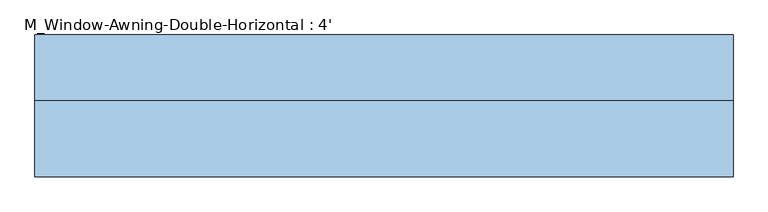
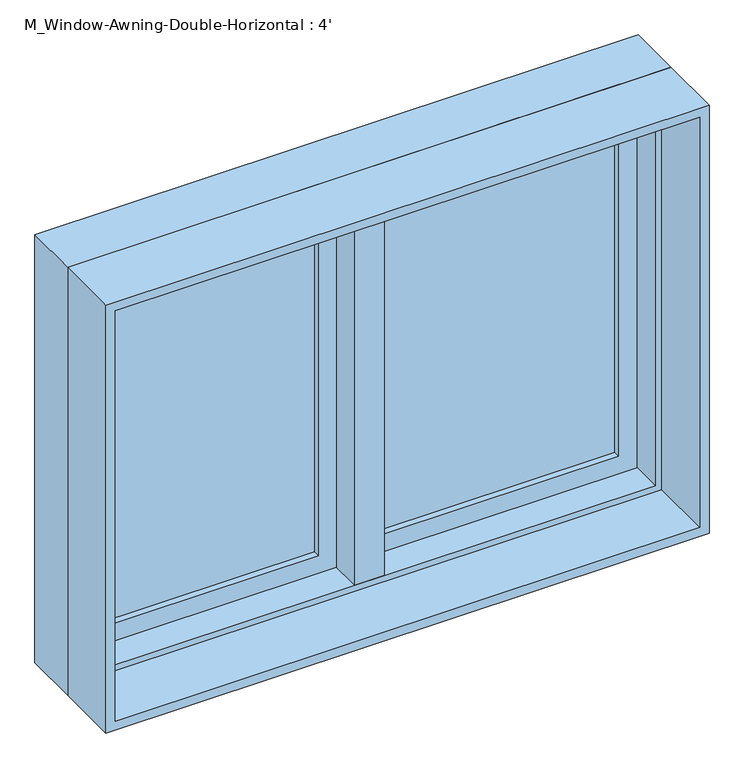
"""IFC4 building model written with IfcOpenShell, lengths in millimetres: window geometry, M_Window-Awning-Double-Horizontal : 4'."""

from ifc_helpers import new_model, si_unit, frame, origin, place, context, project, spatial, polyline, outline, extrude, faceted_brep, source, transform, mapped, element, save


def m_window_awning_double_horizontal_4_0c6a2509(model_context):
    return source(origin(), model_context, "Body", "SolidModel", [
        faceted_brep([(577.85, 82.55, 1782.65), (577.85, 19.05, 1782.65), (-577.85, 19.05, 1782.65), (-577.85, 82.55, 1782.65), (596.9, 133.35, 1801.7), (596.9, 82.55, 1801.7), (-596.9, 82.55, 1801.7), (-596.9, 133.35, 1801.7), (609.6, 19.05, 1814.4), (609.6, 133.35, 1814.4), (-609.6, 133.35, 1814.4), (-609.6, 19.05, 1814.4), (-577.85, 19.05, 931.75), (-577.85, 82.55, 931.75), (-596.9, 82.55, 912.7), (-596.9, 133.35, 912.7), (-609.6, 133.35, 900.0), (-609.6, 19.05, 900.0), (577.85, 19.05, 931.75), (577.85, 82.55, 931.75), (596.9, 82.55, 912.7), (596.9, 133.35, 912.7), (609.6, 133.35, 900.0), (609.6, 19.05, 900.0)], [[[0, 1, 2, 3]], [[4, 5, 6, 7]], [[8, 9, 10, 11]], [[3, 2, 12, 13]], [[7, 6, 14, 15]], [[11, 10, 16, 17]], [[13, 12, 18, 19]], [[15, 14, 20, 21]], [[17, 16, 22, 23]], [[11, 17, 23, 8], [1, 18, 12, 2]], [[19, 18, 1, 0]], [[5, 20, 14, 6], [3, 13, 19, 0]], [[21, 20, 5, 4]], [[23, 22, 9, 8]], [[9, 22, 16, 10], [7, 15, 21, 4]]]),
        extrude(outline(polyline([(1814.4, -609.6), (900.0, -609.6), (900.0, 609.6), (1814.4, 609.6), (1814.4, -609.6)]), holes=[polyline([(1795.35, 590.55), (919.05, 590.55), (919.05, -590.55), (1795.35, -590.55), (1795.35, 590.55)])]), frame((0.0, -114.3, 0.0), z_axis=(0.0, 1.0, 0.0), x_axis=(0.0, 0.0, 1.0)), (0.0, 0.0, 1.0), 133.35),
        extrude(outline(polyline([(912.7, 596.9), (1801.7, 596.9), (1801.7, 9.525), (912.7, 9.525), (912.7, 596.9)]), holes=[polyline([(969.85, 66.675), (1744.55, 66.675), (1744.55, 539.75), (969.85, 539.75), (969.85, 66.675)])]), frame((0.0, 82.55, 0.0), z_axis=(0.0, 1.0, 0.0), x_axis=(0.0, 0.0, 1.0)), (0.0, 0.0, 1.0), 44.45),
        extrude(outline(polyline([(1801.7, -596.9), (912.7, -596.9), (912.7, -9.525), (1801.7, -9.525), (1801.7, -596.9)]), holes=[polyline([(1744.55, -66.675), (969.85, -66.675), (969.85, -539.75), (1744.55, -539.75), (1744.55, -66.675)])]), frame((0.0, 82.55, 0.0), z_axis=(0.0, 1.0, 0.0), x_axis=(0.0, 0.0, 1.0)), (0.0, 0.0, 1.0), 44.45),
        extrude(outline(polyline([(539.75, 114.3), (539.75, 107.95), (66.675, 107.95), (66.675, 114.3), (539.75, 114.3)])), frame((0.0, 0.0, 969.85), z_axis=(0.0, 0.0, 1.0), x_axis=(1.0, 0.0, 0.0)), (0.0, 0.0, 1.0), 774.7),
        extrude(outline(polyline([(66.675, 95.25), (66.675, 101.6), (539.75, 101.6), (539.75, 95.25), (66.675, 95.25)])), frame((0.0, 0.0, 969.85), z_axis=(0.0, 0.0, 1.0), x_axis=(1.0, 0.0, 0.0)), (0.0, 0.0, 1.0), 774.7),
        extrude(outline(polyline([(-66.675, 114.3), (-66.675, 107.95), (-539.75, 107.95), (-539.75, 114.3), (-66.675, 114.3)])), frame((0.0, 0.0, 969.85), z_axis=(0.0, 0.0, 1.0), x_axis=(1.0, 0.0, 0.0)), (0.0, 0.0, 1.0), 774.7),
        extrude(outline(polyline([(-539.75, 95.25), (-539.75, 101.6), (-66.675, 101.6), (-66.675, 95.25), (-539.75, 95.25)])), frame((0.0, 0.0, 969.85), z_axis=(0.0, 0.0, 1.0), x_axis=(1.0, 0.0, 0.0)), (0.0, 0.0, 1.0), 774.7),
        faceted_brep([(9.525, 133.35, 1801.7), (-9.525, 133.35, 1801.7), (-9.525, 82.55, 1801.7), (9.525, 82.55, 1801.7), (9.525, 133.35, 912.7), (9.525, 82.55, 912.7), (-9.525, 82.55, 912.7), (-9.525, 133.35, 912.7), (-9.525, 82.55, 931.75), (-9.525, 82.55, 1782.65), (-30.1625, 82.55, 931.75), (-30.1625, 82.55, 1782.65), (-30.1625, 19.05, 931.75), (-30.1625, 19.05, 1782.65), (30.1625, 19.05, 931.75), (30.1625, 19.05, 1782.65), (30.1625, 82.55, 931.75), (30.1625, 82.55, 1782.65), (9.525, 82.55, 931.75), (9.525, 82.55, 1782.65)], [[[0, 1, 2, 3]], [[4, 5, 6, 7]], [[1, 0, 4, 7]], [[2, 1, 7, 6, 8, 9]], [[9, 8, 10, 11]], [[11, 10, 12, 13]], [[13, 12, 14, 15]], [[15, 14, 16, 17]], [[17, 16, 18, 19]], [[0, 3, 19, 18, 5, 4]], [[18, 8, 6, 5]], [[9, 19, 3, 2]], [[8, 18, 16, 14, 12, 10]], [[19, 9, 11, 13, 15, 17]]]),
    ])


if __name__ == "__main__":
    model = new_model("IFC4")
    model_context = context("Model", 3, world=origin())
    ifc_project = project(units=[si_unit("LENGTHUNIT", "METRE", prefix="MILLI")], contexts=[model_context])
    site = spatial("IfcSite", under=ifc_project)
    building = spatial("IfcBuilding", under=site)
    placement = place(None, origin())
    m_window_awning_double_horizontal_4_shape = m_window_awning_double_horizontal_4_0c6a2509(model_context)
    element("IfcWindow", 1, ObjectType="M_Window-Awning-Double-Horizontal : 4'", at=placement, inside=building, context=model_context, shape_type="MappedRepresentation", body=[
        mapped(m_window_awning_double_horizontal_4_shape, transform((0.0, 0.0, 0.0), x_axis=(1.0, 0.0, 0.0), y_axis=(0.0, 1.0, 0.0), z_axis=(0.0, 0.0, 1.0))),
    ])
    save(model, "model.ifc")

# Revit data of these elements
# Type "M_Window-Awning-Double-Horizontal : 4'"
#   Type Mark = "21"
#   Fire Rating = "0.5h"
#   Assembly Code = "B2020100"
#   Analytic Construction = "Double glazing - domestic"
#   Window Inset [instance default] = 0' - 0"
#   Wall Thickness [instance default] = 0' - 5.90551"
#   Interior Wall Closure [instance default] = 0' - 2.15551"
#   Half Width = 2' - 0"
#   Visual Light Transmittance = 0.81
#   Thermal Resistance (R) = 1.8146 (h·ft²·°F)/BTU
#   Solar Heat Gain Coefficient = 0.76
#   Rough Width = 4' - 0.59055"
#   Rough Height = 3' - 0.59055"
#   Height = 3' - 0"
#   Heat Transfer Coefficient (U) = 0.5511 BTU/(h·ft²·°F)
#   Frame Extension [instance default] = 0' - 0 1/4"
#   Exterior Wall Closure [instance default] = 0' - 1 1/4"
#   Extension Jamb [instance default] = 0' - 2.15551"
#   Default Sill Height = 2' - 11.43307"
#   Width = 4' - 0"
#   Muntin Visibility = yes
#   Interior Trim Visibility [instance default] = yes
#   Exterior Trim Visibility [instance default] = yes
#   Extension Jamb Visibility [instance default] = yes
#   Interior Trim Material = Wood - Stained
#   Muntin Pattern = M_Muntin Pattern_2x2 : M_Muntin Pattern_2x2
#   Interior Trim = M_Trim-Window-Interior-Flat : Picture Frame
#   Interior Frame Material = Wood - Stained
#   Glass Panel Material = Glass
#   Exterior Trim Material = Clad - White
#   Exterior Trim = M_Trim-Window-Exterior-Flat : with Sill
#   Exterior Frame Material = Clad - White
#   Wall Closure = (empty or 0)
# Element 1 (IfcWindow, "M_Window-Awning-Double-Horizontal : 4'")
#   Wall Thickness = 0' - 9"
#   Extension Jamb = 0' - 5 1/4"
#   Materials on its faces: "Wood - Stained", "Glass", "Clad - White"
# Materials
#   "Wood - Stained": class "Wood", colour RGB 224 178 126, transparency 0, Cost = 0
#   "Glass": class "Glass", colour RGB 0 128 192, transparency 0.75, Description = "Soda Lime Glass", Cost = 0
#   "Clad - White": class "Wood", colour RGB 242 242 238, transparency 0, Cost = 0
